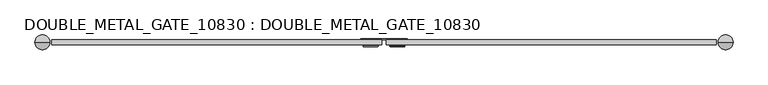
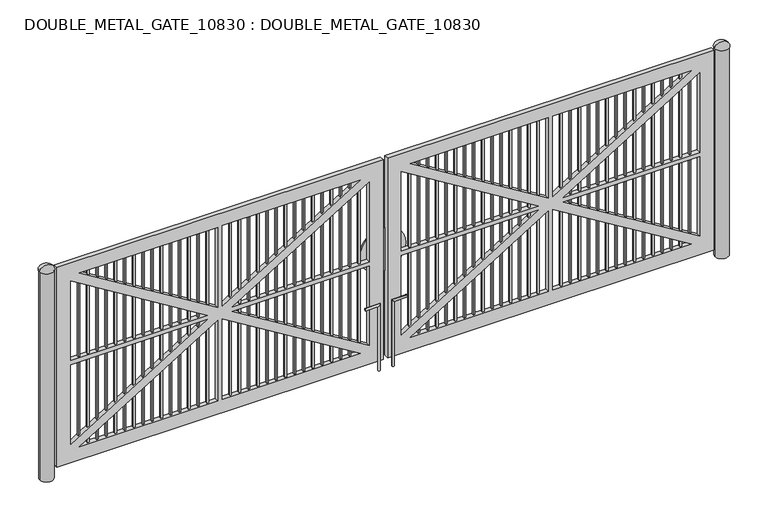
"""IFC4 building model written with IfcOpenShell, lengths in millimetres: proxy geometry, DOUBLE_METAL_GATE_10830 : DOUBLE_METAL_GATE_10830."""

from ifc_helpers import new_model, si_unit, point, frame, frame_2d, origin, origin_with_axes, place, context, project, spatial, polyline, circle_curve, ellipse_curve, trimmed, segment, composite_curve, outline, extrude, source, transform, mapped, element, save
from ifc_brep_helpers import plane_surface, cylinder_surface, revolved_surface, advanced_brep


def double_metal_gate_10830_double_metal_gate_10830_28153ce0(model_context):
    return source(origin(), model_context, "Body", "SolidModel", [
        extrude(outline(composite_curve([segment(trimmed(circle_curve(frame_2d((-4495.8, 76.2)), 76.2), [point((-4572.0, 76.2))], [point((-4419.6, 76.2))], False, "CARTESIAN"), True, "CONTINUOUS"), segment(trimmed(circle_curve(frame_2d((-4495.8, 76.2)), 76.2), [point((-4419.6, 76.2))], [point((-4572.0, 76.2))], False, "CARTESIAN"), True, "CONTINUOUS")], self_intersect=False)), origin_with_axes(), (0.0, 0.0, 1.0), 2438.4),
        advanced_brep(
        [(-4495.8, 76.2, 2489.2), (-4414.8872266, 76.2, 2438.4), (-4576.7127734, 76.2, 2438.4), (-4495.8, 76.2, 2438.4)],
        [
            (0, 1, circle_curve(frame((-4491.2496493, 76.2, 2406.6099024), z_axis=(0.0, 1.0, 0.0), x_axis=(-1.0, 0.0, 0.0)), 82.7153547)),
            (1, 2, circle_curve(frame((-4495.8, 76.2, 2438.4), z_axis=(0.0, 0.0, 1.0), x_axis=(1.0, 0.0, 0.0)), 80.9127734)),
            (2, 0, circle_curve(frame((-4500.3503507, 76.2, 2406.6099024), z_axis=(0.0, 1.0, 0.0), x_axis=(1.0, 0.0, 0.0)), 82.7153547)),
            (2, 1, circle_curve(frame((-4495.8, 76.2, 2438.4), z_axis=(0.0, 0.0, 1.0), x_axis=(1.0, 0.0, 0.0)), 80.9127734)),
            (1, 3),
            (3, 2),
        ],
        [
            revolved_surface(trimmed(ellipse_curve(frame((-4491.2496493, 76.2, 2406.6099024), z_axis=(0.0, -1.0, 0.0), x_axis=(-1.0, 0.0, 0.0)), 82.7153547, 82.7153547), [point((-4414.8872266, 76.2, 2438.4))], [point((-4495.8, 76.2, 2489.2))], True, "CARTESIAN"), (-4495.8, 76.2, 2438.4), (0.0, 0.0, 1.0)),
            plane_surface(frame((-4495.8, 76.2, 2438.4), z_axis=(0.0, 0.0, -1.0), x_axis=(1.0, 0.0, 0.0))),
        ],
        [
            (0, [[1, 2, 3]]),
            (0, [[-3, 4, -1]]),
            (1, [[-2, 5, 6]]),
            (1, [[-4, -6, -5]]),
        ],
    ),
        advanced_brep(
        [(2971.8, 76.2, 2489.2), (3052.7127734, 76.2, 2438.4), (2890.8872266, 76.2, 2438.4), (2971.8, 76.2, 2438.4)],
        [
            (0, 1, circle_curve(frame((2976.3503507, 76.2, 2406.6099024), z_axis=(0.0, 1.0, 0.0), x_axis=(-1.0, 0.0, 0.0)), 82.7153547)),
            (1, 2, circle_curve(frame((2971.8, 76.2, 2438.4), z_axis=(0.0, 0.0, 1.0), x_axis=(1.0, 0.0, 0.0)), 80.9127734)),
            (2, 0, circle_curve(frame((2967.2496493, 76.2, 2406.6099024), z_axis=(0.0, 1.0, 0.0), x_axis=(1.0, 0.0, 0.0)), 82.7153547)),
            (2, 1, circle_curve(frame((2971.8, 76.2, 2438.4), z_axis=(0.0, 0.0, 1.0), x_axis=(1.0, 0.0, 0.0)), 80.9127734)),
            (1, 3),
            (3, 2),
        ],
        [
            revolved_surface(trimmed(ellipse_curve(frame((2976.3503507, 76.2, 2406.6099024), z_axis=(0.0, -1.0, 0.0), x_axis=(-1.0, 0.0, 0.0)), 82.7153547, 82.7153547), [point((3052.7127734, 76.2, 2438.4))], [point((2971.8, 76.2, 2489.2))], True, "CARTESIAN"), (2971.8, 76.2, 2438.4), (0.0, 0.0, 1.0)),
            plane_surface(frame((2971.8, 76.2, 2438.4), z_axis=(0.0, 0.0, -1.0), x_axis=(1.0, 0.0, 0.0))),
        ],
        [
            (0, [[1, 2, 3]]),
            (0, [[-3, 4, -1]]),
            (1, [[-2, 5, 6]]),
            (1, [[-4, -6, -5]]),
        ],
    ),
        extrude(outline(composite_curve([segment(trimmed(circle_curve(frame_2d((2971.8, 76.2)), 76.2), [point((3048.0, 76.2))], [point((2895.6, 76.2))], False, "CARTESIAN"), True, "CONTINUOUS"), segment(trimmed(circle_curve(frame_2d((2971.8, 76.2)), 76.2), [point((2895.6, 76.2))], [point((3048.0, 76.2))], False, "CARTESIAN"), True, "CONTINUOUS")], self_intersect=False)), origin_with_axes(), (0.0, 0.0, 1.0), 2438.4),
        extrude(outline(polyline([(101.6, -787.4), (2438.4, -787.4), (2438.4, -4394.2), (101.6, -4394.2), (101.6, -787.4)]), holes=[polyline([(2286.0, -1036.7285433), (1345.2791035, -2565.4), (2286.0, -2565.4), (2286.0, -1036.7285433)]), polyline([(2226.3516657, -4241.8), (1295.4, -2729.0035433), (1295.4, -4241.8), (2226.3516657, -4241.8)]), polyline([(2286.0, -2616.2), (1345.2791035, -2616.2), (2286.0, -4144.8714567), (2286.0, -2616.2)]), polyline([(1244.6, -4241.8), (1244.6, -2729.0035433), (313.6483343, -4241.8), (1244.6, -4241.8)]), polyline([(254.0, -2565.4), (1194.7208965, -2565.4), (254.0, -1036.7285433), (254.0, -2565.4)]), polyline([(1295.4, -939.8), (1295.4, -2452.5964567), (2226.3516657, -939.8), (1295.4, -939.8)]), polyline([(1244.6, -2452.5964567), (1244.6, -939.8), (313.6483343, -939.8), (1244.6, -2452.5964567)]), polyline([(1194.7208965, -2616.2), (254.0, -2616.2), (254.0, -4144.8714567), (1194.7208965, -2616.2)])]), frame((0.0, 50.8, 0.0), z_axis=(0.0, 1.0, 0.0), x_axis=(0.0, 0.0, 1.0)), (0.0, 0.0, 1.0), 50.8),
        extrude(outline(polyline([(-4130.675, 66.675), (-4149.725, 66.675), (-4149.725, 85.725), (-4130.675, 85.725), (-4130.675, 66.675)])), frame((0.0, 0.0, 254.0), z_axis=(0.0, 0.0, 1.0), x_axis=(1.0, 0.0, 0.0)), (0.0, 0.0, 1.0), 2032.0),
        extrude(outline(polyline([(-4029.075, 66.675), (-4048.125, 66.675), (-4048.125, 85.725), (-4029.075, 85.725), (-4029.075, 66.675)])), frame((0.0, 0.0, 254.0), z_axis=(0.0, 0.0, 1.0), x_axis=(1.0, 0.0, 0.0)), (0.0, 0.0, 1.0), 2032.0),
        extrude(outline(polyline([(-3927.475, 66.675), (-3946.525, 66.675), (-3946.525, 85.725), (-3927.475, 85.725), (-3927.475, 66.675)])), frame((0.0, 0.0, 254.0), z_axis=(0.0, 0.0, 1.0), x_axis=(1.0, 0.0, 0.0)), (0.0, 0.0, 1.0), 2032.0),
        extrude(outline(polyline([(-3825.875, 66.675), (-3844.925, 66.675), (-3844.925, 85.725), (-3825.875, 85.725), (-3825.875, 66.675)])), frame((0.0, 0.0, 254.0), z_axis=(0.0, 0.0, 1.0), x_axis=(1.0, 0.0, 0.0)), (0.0, 0.0, 1.0), 2032.0),
        extrude(outline(polyline([(-3724.275, 66.675), (-3743.325, 66.675), (-3743.325, 85.725), (-3724.275, 85.725), (-3724.275, 66.675)])), frame((0.0, 0.0, 254.0), z_axis=(0.0, 0.0, 1.0), x_axis=(1.0, 0.0, 0.0)), (0.0, 0.0, 1.0), 2032.0),
        extrude(outline(polyline([(-3622.675, 66.675), (-3641.725, 66.675), (-3641.725, 85.725), (-3622.675, 85.725), (-3622.675, 66.675)])), frame((0.0, 0.0, 254.0), z_axis=(0.0, 0.0, 1.0), x_axis=(1.0, 0.0, 0.0)), (0.0, 0.0, 1.0), 2032.0),
        extrude(outline(polyline([(-3521.075, 66.675), (-3540.125, 66.675), (-3540.125, 85.725), (-3521.075, 85.725), (-3521.075, 66.675)])), frame((0.0, 0.0, 254.0), z_axis=(0.0, 0.0, 1.0), x_axis=(1.0, 0.0, 0.0)), (0.0, 0.0, 1.0), 2032.0),
        extrude(outline(polyline([(-3419.475, 66.675), (-3438.525, 66.675), (-3438.525, 85.725), (-3419.475, 85.725), (-3419.475, 66.675)])), frame((0.0, 0.0, 254.0), z_axis=(0.0, 0.0, 1.0), x_axis=(1.0, 0.0, 0.0)), (0.0, 0.0, 1.0), 2032.0),
        extrude(outline(polyline([(-3317.875, 66.675), (-3336.925, 66.675), (-3336.925, 85.725), (-3317.875, 85.725), (-3317.875, 66.675)])), frame((0.0, 0.0, 254.0), z_axis=(0.0, 0.0, 1.0), x_axis=(1.0, 0.0, 0.0)), (0.0, 0.0, 1.0), 2032.0),
        extrude(outline(polyline([(-3216.275, 66.675), (-3235.325, 66.675), (-3235.325, 85.725), (-3216.275, 85.725), (-3216.275, 66.675)])), frame((0.0, 0.0, 254.0), z_axis=(0.0, 0.0, 1.0), x_axis=(1.0, 0.0, 0.0)), (0.0, 0.0, 1.0), 2032.0),
        extrude(outline(polyline([(-3114.675, 66.675), (-3133.725, 66.675), (-3133.725, 85.725), (-3114.675, 85.725), (-3114.675, 66.675)])), frame((0.0, 0.0, 254.0), z_axis=(0.0, 0.0, 1.0), x_axis=(1.0, 0.0, 0.0)), (0.0, 0.0, 1.0), 2032.0),
        extrude(outline(polyline([(-3013.075, 66.675), (-3032.125, 66.675), (-3032.125, 85.725), (-3013.075, 85.725), (-3013.075, 66.675)])), frame((0.0, 0.0, 254.0), z_axis=(0.0, 0.0, 1.0), x_axis=(1.0, 0.0, 0.0)), (0.0, 0.0, 1.0), 2032.0),
        extrude(outline(polyline([(-2911.475, 66.675), (-2930.525, 66.675), (-2930.525, 85.725), (-2911.475, 85.725), (-2911.475, 66.675)])), frame((0.0, 0.0, 254.0), z_axis=(0.0, 0.0, 1.0), x_axis=(1.0, 0.0, 0.0)), (0.0, 0.0, 1.0), 2032.0),
        extrude(outline(polyline([(-2809.875, 66.675), (-2828.925, 66.675), (-2828.925, 85.725), (-2809.875, 85.725), (-2809.875, 66.675)])), frame((0.0, 0.0, 254.0), z_axis=(0.0, 0.0, 1.0), x_axis=(1.0, 0.0, 0.0)), (0.0, 0.0, 1.0), 2032.0),
        extrude(outline(polyline([(-2708.275, 66.675), (-2727.325, 66.675), (-2727.325, 85.725), (-2708.275, 85.725), (-2708.275, 66.675)])), frame((0.0, 0.0, 254.0), z_axis=(0.0, 0.0, 1.0), x_axis=(1.0, 0.0, 0.0)), (0.0, 0.0, 1.0), 2032.0),
        extrude(outline(polyline([(-2454.275, 66.675), (-2473.325, 66.675), (-2473.325, 85.725), (-2454.275, 85.725), (-2454.275, 66.675)])), frame((0.0, 0.0, 254.0), z_axis=(0.0, 0.0, 1.0), x_axis=(1.0, 0.0, 0.0)), (0.0, 0.0, 1.0), 2032.0),
        extrude(outline(polyline([(-2352.675, 66.675), (-2371.725, 66.675), (-2371.725, 85.725), (-2352.675, 85.725), (-2352.675, 66.675)])), frame((0.0, 0.0, 254.0), z_axis=(0.0, 0.0, 1.0), x_axis=(1.0, 0.0, 0.0)), (0.0, 0.0, 1.0), 2032.0),
        extrude(outline(polyline([(-2251.075, 66.675), (-2270.125, 66.675), (-2270.125, 85.725), (-2251.075, 85.725), (-2251.075, 66.675)])), frame((0.0, 0.0, 254.0), z_axis=(0.0, 0.0, 1.0), x_axis=(1.0, 0.0, 0.0)), (0.0, 0.0, 1.0), 2032.0),
        extrude(outline(polyline([(-2149.475, 66.675), (-2168.525, 66.675), (-2168.525, 85.725), (-2149.475, 85.725), (-2149.475, 66.675)])), frame((0.0, 0.0, 254.0), z_axis=(0.0, 0.0, 1.0), x_axis=(1.0, 0.0, 0.0)), (0.0, 0.0, 1.0), 2032.0),
        extrude(outline(polyline([(-2047.875, 66.675), (-2066.925, 66.675), (-2066.925, 85.725), (-2047.875, 85.725), (-2047.875, 66.675)])), frame((0.0, 0.0, 254.0), z_axis=(0.0, 0.0, 1.0), x_axis=(1.0, 0.0, 0.0)), (0.0, 0.0, 1.0), 2032.0),
        extrude(outline(polyline([(-1946.275, 66.675), (-1965.325, 66.675), (-1965.325, 85.725), (-1946.275, 85.725), (-1946.275, 66.675)])), frame((0.0, 0.0, 254.0), z_axis=(0.0, 0.0, 1.0), x_axis=(1.0, 0.0, 0.0)), (0.0, 0.0, 1.0), 2032.0),
        extrude(outline(polyline([(-1844.675, 66.675), (-1863.725, 66.675), (-1863.725, 85.725), (-1844.675, 85.725), (-1844.675, 66.675)])), frame((0.0, 0.0, 254.0), z_axis=(0.0, 0.0, 1.0), x_axis=(1.0, 0.0, 0.0)), (0.0, 0.0, 1.0), 2032.0),
        extrude(outline(polyline([(-1743.075, 66.675), (-1762.125, 66.675), (-1762.125, 85.725), (-1743.075, 85.725), (-1743.075, 66.675)])), frame((0.0, 0.0, 254.0), z_axis=(0.0, 0.0, 1.0), x_axis=(1.0, 0.0, 0.0)), (0.0, 0.0, 1.0), 2032.0),
        extrude(outline(polyline([(-1641.475, 66.675), (-1660.525, 66.675), (-1660.525, 85.725), (-1641.475, 85.725), (-1641.475, 66.675)])), frame((0.0, 0.0, 254.0), z_axis=(0.0, 0.0, 1.0), x_axis=(1.0, 0.0, 0.0)), (0.0, 0.0, 1.0), 2032.0),
        extrude(outline(polyline([(-1539.875, 66.675), (-1558.925, 66.675), (-1558.925, 85.725), (-1539.875, 85.725), (-1539.875, 66.675)])), frame((0.0, 0.0, 254.0), z_axis=(0.0, 0.0, 1.0), x_axis=(1.0, 0.0, 0.0)), (0.0, 0.0, 1.0), 2032.0),
        extrude(outline(polyline([(-1438.275, 66.675), (-1457.325, 66.675), (-1457.325, 85.725), (-1438.275, 85.725), (-1438.275, 66.675)])), frame((0.0, 0.0, 254.0), z_axis=(0.0, 0.0, 1.0), x_axis=(1.0, 0.0, 0.0)), (0.0, 0.0, 1.0), 2032.0),
        extrude(outline(polyline([(-1336.675, 66.675), (-1355.725, 66.675), (-1355.725, 85.725), (-1336.675, 85.725), (-1336.675, 66.675)])), frame((0.0, 0.0, 254.0), z_axis=(0.0, 0.0, 1.0), x_axis=(1.0, 0.0, 0.0)), (0.0, 0.0, 1.0), 2032.0),
        extrude(outline(polyline([(-1235.075, 66.675), (-1254.125, 66.675), (-1254.125, 85.725), (-1235.075, 85.725), (-1235.075, 66.675)])), frame((0.0, 0.0, 254.0), z_axis=(0.0, 0.0, 1.0), x_axis=(1.0, 0.0, 0.0)), (0.0, 0.0, 1.0), 2032.0),
        extrude(outline(polyline([(-1133.475, 66.675), (-1152.525, 66.675), (-1152.525, 85.725), (-1133.475, 85.725), (-1133.475, 66.675)])), frame((0.0, 0.0, 254.0), z_axis=(0.0, 0.0, 1.0), x_axis=(1.0, 0.0, 0.0)), (0.0, 0.0, 1.0), 2032.0),
        extrude(outline(polyline([(-1031.875, 66.675), (-1050.925, 66.675), (-1050.925, 85.725), (-1031.875, 85.725), (-1031.875, 66.675)])), frame((0.0, 0.0, 254.0), z_axis=(0.0, 0.0, 1.0), x_axis=(1.0, 0.0, 0.0)), (0.0, 0.0, 1.0), 2032.0),
        extrude(outline(polyline([(101.6, -736.6), (101.6, 2870.2), (2438.4, 2870.2), (2438.4, -736.6), (101.6, -736.6)]), holes=[polyline([(2286.0, 1092.2), (2286.0, 2620.8714567), (1345.2791035, 1092.2), (2286.0, 1092.2)]), polyline([(1295.4, -584.2), (2226.3516657, -584.2), (1295.4, 928.5964567), (1295.4, -584.2)]), polyline([(254.0, 1041.4), (254.0, -487.2714567), (1194.7208965, 1041.4), (254.0, 1041.4)]), polyline([(1244.6, 2717.8), (313.6483343, 2717.8), (1244.6, 1205.0035433), (1244.6, 2717.8)]), polyline([(1194.7208965, 1092.2), (254.0, 2620.8714567), (254.0, 1092.2), (1194.7208965, 1092.2)]), polyline([(1244.6, 928.5964567), (313.6483343, -584.2), (1244.6, -584.2), (1244.6, 928.5964567)]), polyline([(2286.0, -487.2714567), (2286.0, 1041.4), (1345.2791035, 1041.4), (2286.0, -487.2714567)]), polyline([(2226.3516657, 2717.8), (1295.4, 2717.8), (1295.4, 1205.0035433), (2226.3516657, 2717.8)])]), frame((0.0, 50.8, 0.0), z_axis=(0.0, 1.0, 0.0), x_axis=(0.0, 0.0, 1.0)), (0.0, 0.0, 1.0), 50.8),
        extrude(outline(composite_curve([segment(trimmed(circle_curve(frame_2d((1342.973777, -762.0)), 254.0), [point((1342.973777, -1016.0))], [point((1342.973777, -508.0))], False, "CARTESIAN"), True, "CONTINUOUS"), segment(trimmed(circle_curve(frame_2d((1342.973777, -762.0)), 254.0), [point((1342.973777, -508.0))], [point((1342.973777, -1016.0))], False, "CARTESIAN"), True, "CONTINUOUS")], self_intersect=False)), frame((0.0, 101.6, 0.0), z_axis=(0.0, 1.0, 0.0), x_axis=(0.0, 0.0, 1.0)), (0.0, 0.0, 1.0), 12.7),
        extrude(outline(polyline([(2606.675, 66.675), (2606.675, 85.725), (2625.725, 85.725), (2625.725, 66.675), (2606.675, 66.675)])), frame((0.0, 0.0, 254.0), z_axis=(0.0, 0.0, 1.0), x_axis=(1.0, 0.0, 0.0)), (0.0, 0.0, 1.0), 2032.0),
        extrude(outline(polyline([(2505.075, 66.675), (2505.075, 85.725), (2524.125, 85.725), (2524.125, 66.675), (2505.075, 66.675)])), frame((0.0, 0.0, 254.0), z_axis=(0.0, 0.0, 1.0), x_axis=(1.0, 0.0, 0.0)), (0.0, 0.0, 1.0), 2032.0),
        extrude(outline(polyline([(2403.475, 66.675), (2403.475, 85.725), (2422.525, 85.725), (2422.525, 66.675), (2403.475, 66.675)])), frame((0.0, 0.0, 254.0), z_axis=(0.0, 0.0, 1.0), x_axis=(1.0, 0.0, 0.0)), (0.0, 0.0, 1.0), 2032.0),
        extrude(outline(polyline([(2301.875, 66.675), (2301.875, 85.725), (2320.925, 85.725), (2320.925, 66.675), (2301.875, 66.675)])), frame((0.0, 0.0, 254.0), z_axis=(0.0, 0.0, 1.0), x_axis=(1.0, 0.0, 0.0)), (0.0, 0.0, 1.0), 2032.0),
        extrude(outline(polyline([(2200.275, 66.675), (2200.275, 85.725), (2219.325, 85.725), (2219.325, 66.675), (2200.275, 66.675)])), frame((0.0, 0.0, 254.0), z_axis=(0.0, 0.0, 1.0), x_axis=(1.0, 0.0, 0.0)), (0.0, 0.0, 1.0), 2032.0),
        extrude(outline(polyline([(2098.675, 66.675), (2098.675, 85.725), (2117.725, 85.725), (2117.725, 66.675), (2098.675, 66.675)])), frame((0.0, 0.0, 254.0), z_axis=(0.0, 0.0, 1.0), x_axis=(1.0, 0.0, 0.0)), (0.0, 0.0, 1.0), 2032.0),
        extrude(outline(polyline([(1997.075, 66.675), (1997.075, 85.725), (2016.125, 85.725), (2016.125, 66.675), (1997.075, 66.675)])), frame((0.0, 0.0, 254.0), z_axis=(0.0, 0.0, 1.0), x_axis=(1.0, 0.0, 0.0)), (0.0, 0.0, 1.0), 2032.0),
        extrude(outline(polyline([(1895.475, 66.675), (1895.475, 85.725), (1914.525, 85.725), (1914.525, 66.675), (1895.475, 66.675)])), frame((0.0, 0.0, 254.0), z_axis=(0.0, 0.0, 1.0), x_axis=(1.0, 0.0, 0.0)), (0.0, 0.0, 1.0), 2032.0),
        extrude(outline(polyline([(1793.875, 66.675), (1793.875, 85.725), (1812.925, 85.725), (1812.925, 66.675), (1793.875, 66.675)])), frame((0.0, 0.0, 254.0), z_axis=(0.0, 0.0, 1.0), x_axis=(1.0, 0.0, 0.0)), (0.0, 0.0, 1.0), 2032.0),
        extrude(outline(polyline([(1692.275, 66.675), (1692.275, 85.725), (1711.325, 85.725), (1711.325, 66.675), (1692.275, 66.675)])), frame((0.0, 0.0, 254.0), z_axis=(0.0, 0.0, 1.0), x_axis=(1.0, 0.0, 0.0)), (0.0, 0.0, 1.0), 2032.0),
        extrude(outline(polyline([(1590.675, 66.675), (1590.675, 85.725), (1609.725, 85.725), (1609.725, 66.675), (1590.675, 66.675)])), frame((0.0, 0.0, 254.0), z_axis=(0.0, 0.0, 1.0), x_axis=(1.0, 0.0, 0.0)), (0.0, 0.0, 1.0), 2032.0),
        extrude(outline(polyline([(1489.075, 66.675), (1489.075, 85.725), (1508.125, 85.725), (1508.125, 66.675), (1489.075, 66.675)])), frame((0.0, 0.0, 254.0), z_axis=(0.0, 0.0, 1.0), x_axis=(1.0, 0.0, 0.0)), (0.0, 0.0, 1.0), 2032.0),
        extrude(outline(polyline([(1387.475, 66.675), (1387.475, 85.725), (1406.525, 85.725), (1406.525, 66.675), (1387.475, 66.675)])), frame((0.0, 0.0, 254.0), z_axis=(0.0, 0.0, 1.0), x_axis=(1.0, 0.0, 0.0)), (0.0, 0.0, 1.0), 2032.0),
        extrude(outline(polyline([(1285.875, 66.675), (1285.875, 85.725), (1304.925, 85.725), (1304.925, 66.675), (1285.875, 66.675)])), frame((0.0, 0.0, 254.0), z_axis=(0.0, 0.0, 1.0), x_axis=(1.0, 0.0, 0.0)), (0.0, 0.0, 1.0), 2032.0),
        extrude(outline(polyline([(1184.275, 66.675), (1184.275, 85.725), (1203.325, 85.725), (1203.325, 66.675), (1184.275, 66.675)])), frame((0.0, 0.0, 254.0), z_axis=(0.0, 0.0, 1.0), x_axis=(1.0, 0.0, 0.0)), (0.0, 0.0, 1.0), 2032.0),
        extrude(outline(polyline([(930.275, 66.675), (930.275, 85.725), (949.325, 85.725), (949.325, 66.675), (930.275, 66.675)])), frame((0.0, 0.0, 254.0), z_axis=(0.0, 0.0, 1.0), x_axis=(1.0, 0.0, 0.0)), (0.0, 0.0, 1.0), 2032.0),
        extrude(outline(polyline([(828.675, 66.675), (828.675, 85.725), (847.725, 85.725), (847.725, 66.675), (828.675, 66.675)])), frame((0.0, 0.0, 254.0), z_axis=(0.0, 0.0, 1.0), x_axis=(1.0, 0.0, 0.0)), (0.0, 0.0, 1.0), 2032.0),
        extrude(outline(polyline([(727.075, 66.675), (727.075, 85.725), (746.125, 85.725), (746.125, 66.675), (727.075, 66.675)])), frame((0.0, 0.0, 254.0), z_axis=(0.0, 0.0, 1.0), x_axis=(1.0, 0.0, 0.0)), (0.0, 0.0, 1.0), 2032.0),
        extrude(outline(polyline([(625.475, 66.675), (625.475, 85.725), (644.525, 85.725), (644.525, 66.675), (625.475, 66.675)])), frame((0.0, 0.0, 254.0), z_axis=(0.0, 0.0, 1.0), x_axis=(1.0, 0.0, 0.0)), (0.0, 0.0, 1.0), 2032.0),
        extrude(outline(polyline([(523.875, 66.675), (523.875, 85.725), (542.925, 85.725), (542.925, 66.675), (523.875, 66.675)])), frame((0.0, 0.0, 254.0), z_axis=(0.0, 0.0, 1.0), x_axis=(1.0, 0.0, 0.0)), (0.0, 0.0, 1.0), 2032.0),
        extrude(outline(polyline([(422.275, 66.675), (422.275, 85.725), (441.325, 85.725), (441.325, 66.675), (422.275, 66.675)])), frame((0.0, 0.0, 254.0), z_axis=(0.0, 0.0, 1.0), x_axis=(1.0, 0.0, 0.0)), (0.0, 0.0, 1.0), 2032.0),
        extrude(outline(polyline([(320.675, 66.675), (320.675, 85.725), (339.725, 85.725), (339.725, 66.675), (320.675, 66.675)])), frame((0.0, 0.0, 254.0), z_axis=(0.0, 0.0, 1.0), x_axis=(1.0, 0.0, 0.0)), (0.0, 0.0, 1.0), 2032.0),
        extrude(outline(polyline([(219.075, 66.675), (219.075, 85.725), (238.125, 85.725), (238.125, 66.675), (219.075, 66.675)])), frame((0.0, 0.0, 254.0), z_axis=(0.0, 0.0, 1.0), x_axis=(1.0, 0.0, 0.0)), (0.0, 0.0, 1.0), 2032.0),
        extrude(outline(polyline([(117.475, 66.675), (117.475, 85.725), (136.525, 85.725), (136.525, 66.675), (117.475, 66.675)])), frame((0.0, 0.0, 254.0), z_axis=(0.0, 0.0, 1.0), x_axis=(1.0, 0.0, 0.0)), (0.0, 0.0, 1.0), 2032.0),
        extrude(outline(polyline([(15.875, 66.675), (15.875, 85.725), (34.925, 85.725), (34.925, 66.675), (15.875, 66.675)])), frame((0.0, 0.0, 254.0), z_axis=(0.0, 0.0, 1.0), x_axis=(1.0, 0.0, 0.0)), (0.0, 0.0, 1.0), 2032.0),
        extrude(outline(polyline([(-85.725, 66.675), (-85.725, 85.725), (-66.675, 85.725), (-66.675, 66.675), (-85.725, 66.675)])), frame((0.0, 0.0, 254.0), z_axis=(0.0, 0.0, 1.0), x_axis=(1.0, 0.0, 0.0)), (0.0, 0.0, 1.0), 2032.0),
        extrude(outline(polyline([(-187.325, 66.675), (-187.325, 85.725), (-168.275, 85.725), (-168.275, 66.675), (-187.325, 66.675)])), frame((0.0, 0.0, 254.0), z_axis=(0.0, 0.0, 1.0), x_axis=(1.0, 0.0, 0.0)), (0.0, 0.0, 1.0), 2032.0),
        extrude(outline(polyline([(-288.925, 66.675), (-288.925, 85.725), (-269.875, 85.725), (-269.875, 66.675), (-288.925, 66.675)])), frame((0.0, 0.0, 254.0), z_axis=(0.0, 0.0, 1.0), x_axis=(1.0, 0.0, 0.0)), (0.0, 0.0, 1.0), 2032.0),
        extrude(outline(polyline([(-390.525, 66.675), (-390.525, 85.725), (-371.475, 85.725), (-371.475, 66.675), (-390.525, 66.675)])), frame((0.0, 0.0, 254.0), z_axis=(0.0, 0.0, 1.0), x_axis=(1.0, 0.0, 0.0)), (0.0, 0.0, 1.0), 2032.0),
        extrude(outline(polyline([(-492.125, 66.675), (-492.125, 85.725), (-473.075, 85.725), (-473.075, 66.675), (-492.125, 66.675)])), frame((0.0, 0.0, 254.0), z_axis=(0.0, 0.0, 1.0), x_axis=(1.0, 0.0, 0.0)), (0.0, 0.0, 1.0), 2032.0),
        advanced_brep(
        [(-825.5, 38.1, 0.0), (-850.9, 38.1, 0.0), (-825.5, 38.1, 774.7), (-850.9, 38.1, 749.3), (-990.6, 38.1, 774.7), (-990.6, 38.1, 749.3)],
        [
            (0, 1, circle_curve(frame((-838.2, 38.1, 0.0), z_axis=(0.0, 0.0, -1.0), x_axis=(-1.0, 0.0, 0.0)), 12.7)),
            (1, 0, circle_curve(frame((-838.2, 38.1, 0.0), z_axis=(0.0, 0.0, -1.0), x_axis=(-1.0, 0.0, 0.0)), 12.7)),
            (0, 2),
            (2, 3, ellipse_curve(frame((-838.2, 38.1, 762.0), z_axis=(0.7071067811865457, 0.0, -0.7071067811865493), x_axis=(-0.7071067811865493, 0.0, -0.7071067811865457)), 17.9605122, 12.7)),
            (3, 1),
            (3, 2, ellipse_curve(frame((-838.2, 38.1, 762.0), z_axis=(0.7071067811865457, 0.0, -0.7071067811865493), x_axis=(-0.7071067811865493, 0.0, -0.7071067811865457)), 17.9605122, 12.7)),
            (4, 5, circle_curve(frame((-990.6, 38.1, 762.0), z_axis=(-1.0, 0.0, 0.0), x_axis=(0.0, 0.0, -1.0)), 12.7)),
            (5, 4, circle_curve(frame((-990.6, 38.1, 762.0), z_axis=(-1.0, 0.0, 0.0), x_axis=(0.0, 0.0, -1.0)), 12.7)),
            (2, 4),
            (5, 3),
        ],
        [
            plane_surface(frame((-838.2, 50.8, 0.0), z_axis=(0.0, 0.0, -1.0), x_axis=(0.0, -1.0, 0.0))),
            cylinder_surface(frame((-838.2, 38.1, 0.0), z_axis=(0.0, 0.0, -1.0), x_axis=(-1.0, 0.0, 0.0)), 12.7),
            plane_surface(frame((-990.6, 50.8, 762.0), z_axis=(-1.0, 0.0, 0.0), x_axis=(0.0, -1.0, 0.0))),
            cylinder_surface(frame((-838.2, 38.1, 762.0), z_axis=(1.0, 0.0, 0.0), x_axis=(0.0, 0.0, -1.0)), 12.7),
        ],
        [
            (0, [[1, 2]]),
            (1, [[-1, 3, 4, 5]]),
            (1, [[-2, -5, 6, -3]]),
            (2, [[7, 8]]),
            (3, [[-4, 9, -8, 10]]),
            (3, [[-6, -10, -7, -9]]),
        ],
    ),
        advanced_brep(
        [(-673.1, 38.1, 0.0), (-698.5, 38.1, 0.0), (-698.5, 38.1, 774.7), (-673.1, 38.1, 749.3), (-533.4, 38.1, 749.3), (-533.4, 38.1, 774.7)],
        [
            (0, 1, circle_curve(frame((-685.8, 38.1, 0.0), z_axis=(0.0, 0.0, -1.0), x_axis=(-1.0, 0.0, 0.0)), 12.7)),
            (1, 0, circle_curve(frame((-685.8, 38.1, 0.0), z_axis=(0.0, 0.0, -1.0), x_axis=(-1.0, 0.0, 0.0)), 12.7)),
            (1, 2),
            (2, 3, ellipse_curve(frame((-685.8, 38.1, 762.0), z_axis=(-0.7071067811865601, 0.0, -0.7071067811865349), x_axis=(0.7071067811865349, 0.0, -0.7071067811865601)), 17.9605122, 12.7)),
            (3, 0),
            (3, 2, ellipse_curve(frame((-685.8, 38.1, 762.0), z_axis=(-0.7071067811865601, 0.0, -0.7071067811865349), x_axis=(0.7071067811865349, 0.0, -0.7071067811865601)), 17.9605122, 12.7)),
            (4, 5, circle_curve(frame((-533.4, 38.1, 762.0), z_axis=(1.0, 0.0, 0.0), x_axis=(0.0, 0.0, 1.0)), 12.7)),
            (5, 4, circle_curve(frame((-533.4, 38.1, 762.0), z_axis=(1.0, 0.0, 0.0), x_axis=(0.0, 0.0, 1.0)), 12.7)),
            (2, 5),
            (4, 3),
        ],
        [
            plane_surface(frame((-685.8, 50.8, 0.0), z_axis=(0.0, 0.0, -1.0), x_axis=(0.0, -1.0, 0.0))),
            cylinder_surface(frame((-685.8, 38.1, 0.0), z_axis=(0.0, 0.0, -1.0), x_axis=(-1.0, 0.0, 0.0)), 12.7),
            plane_surface(frame((-533.4, 50.8, 762.0), z_axis=(1.0, 0.0, 0.0), x_axis=(0.0, -1.0, 0.0))),
            cylinder_surface(frame((-685.8, 38.1, 762.0), z_axis=(-1.0, 0.0, 0.0), x_axis=(0.0, 0.0, 1.0)), 12.7),
        ],
        [
            (0, [[1, 2]]),
            (1, [[-2, 3, 4, 5]]),
            (1, [[-1, -5, 6, -3]]),
            (2, [[7, 8]]),
            (3, [[-4, 9, -7, 10]]),
            (3, [[-6, -10, -8, -9]]),
        ],
    ),
    ])


if __name__ == "__main__":
    model = new_model("IFC4")
    model_context = context("Model", 3, world=origin())
    ifc_project = project(units=[si_unit("LENGTHUNIT", "METRE", prefix="MILLI")], contexts=[model_context])
    site = spatial("IfcSite", under=ifc_project)
    building = spatial("IfcBuilding", under=site)
    placement = place(None, origin())
    double_metal_gate_10830_double_metal_gate_10830_shape = double_metal_gate_10830_double_metal_gate_10830_28153ce0(model_context)
    element("IfcBuildingElementProxy", 1, Name="DOUBLE_METAL_GATE_10830 : DOUBLE_METAL_GATE_10830", ObjectType="DOUBLE_METAL_GATE_10830 : DOUBLE_METAL_GATE_10830", at=placement, inside=building, context=model_context, shape_type="MappedRepresentation", body=[
        mapped(double_metal_gate_10830_double_metal_gate_10830_shape, transform((0.0, 0.0, 0.0), x_axis=(1.0, 0.0, 0.0), y_axis=(0.0, 1.0, 0.0), z_axis=(0.0, 0.0, 1.0))),
    ])
    save(model, "model.ifc")

# Revit data of these elements
# Type "DOUBLE_METAL_GATE_10830 : DOUBLE_METAL_GATE_10830"
#   WIDTH [instance default] = 24' - 0"
#   Default Elevation = 0
#   Assembly Code = ""
# Element 1 (IfcBuildingElementProxy, "DOUBLE_METAL_GATE_10830 : DOUBLE_METAL_GATE_10830")
#   Materials on its faces: "Default"
# Materials
#   "Default": colour RGB 127 127 127, transparency 0, Cost = 0
